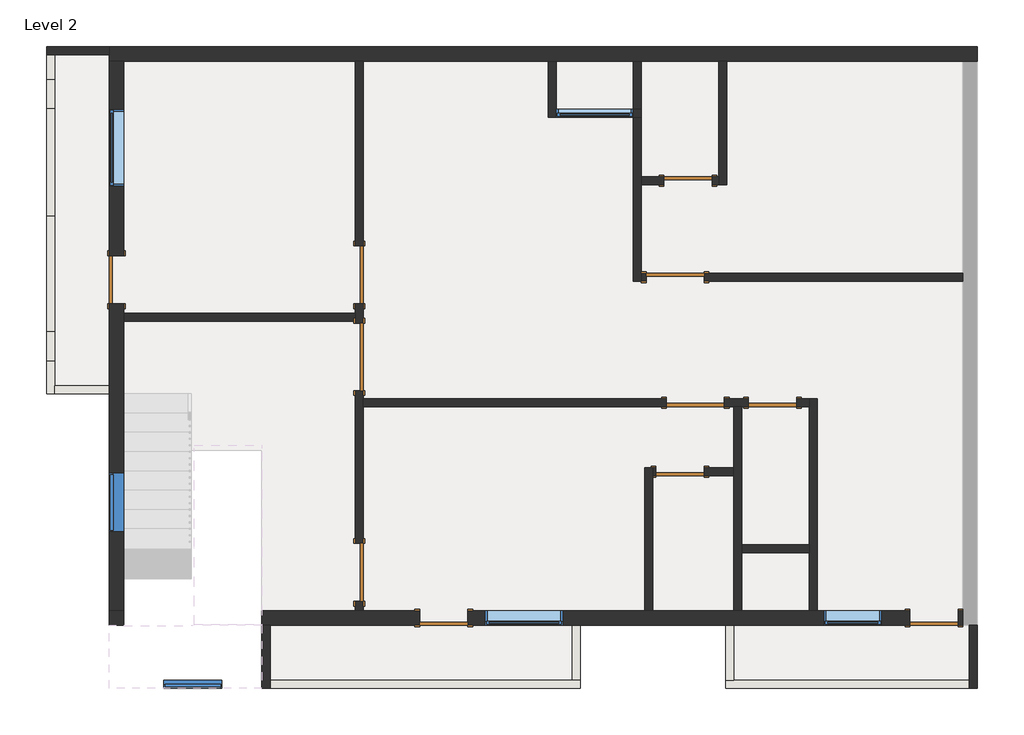
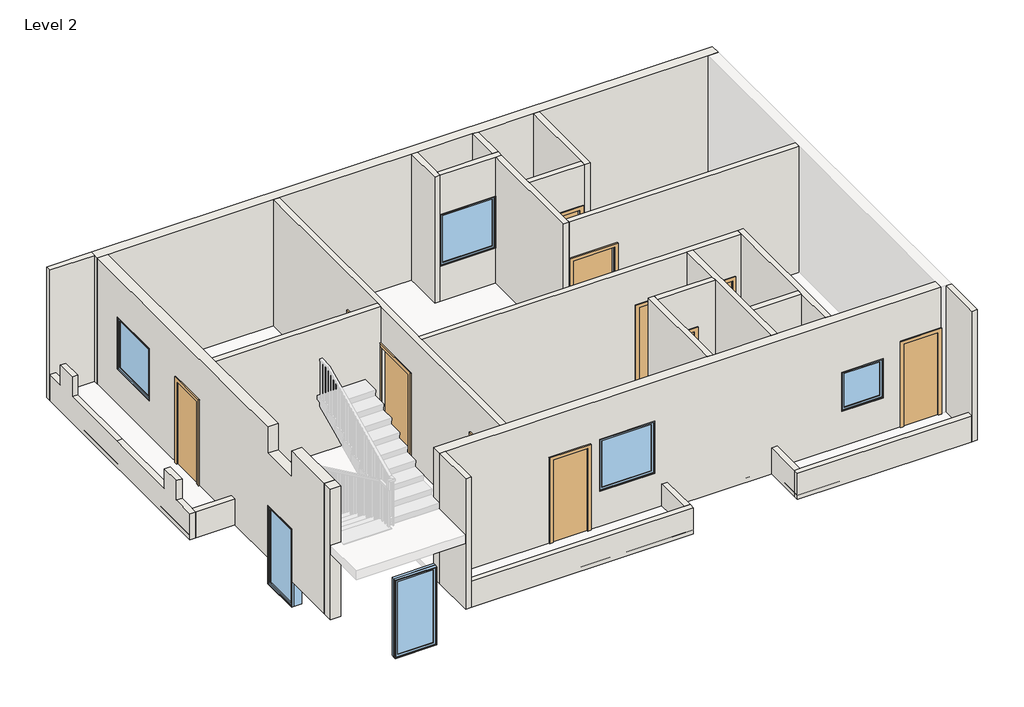
# One storey, part 1 of 2: 28 walls, 11 doors, 6 windows.
"""IFC4 building model written with IfcOpenShell, lengths in millimetres."""

from ifc_helpers import new_model, si_unit, frame, origin, place, context, project, spatial, polyline, outline, extrude, faceted_brep, transform, mapped, element, save
from components import door_1fe7f57d, door_85036156, door_a3eb833a, door_a1797ceb, door_4f94b823, window_6c5853a0, window_7da3115e, window_c796fc87, window_f887c457, window_76f305d9

model = new_model("IFC4")

# Units and contexts
model_context = context("Model", 3, world=origin())
ifc_project = project(units=[si_unit("LENGTHUNIT", "METRE", prefix="MILLI")], contexts=[model_context])

# Site, building, storey
site = spatial("IfcSite", under=ifc_project)
building = spatial("IfcBuilding", under=site)
storey = spatial("IfcBuildingStorey", under=building, Name="Level 2", Elevation=3048.0)

# Doors
placement = place(None, origin())
door_shape = door_1fe7f57d(model_context)
element("IfcDoor", 1, ObjectType="Single-Flush : 30\" x 80\"", at=placement, inside=storey, context=model_context, shape_type="MappedRepresentation", body=[
    mapped(door_shape, transform((-1197.7394758, 10653.5495492, 3048.0), x_axis=(1.0, 0.0, 0.0), y_axis=(0.0, 1.0, 0.0), z_axis=(0.0, 0.0, 1.0))),
])
element("IfcDoor", 2, ObjectType="Single-Flush : 30\" x 80\"", at=placement, inside=storey, context=model_context, shape_type="MappedRepresentation", body=[
    mapped(door_shape, transform((135.7605242, 7148.3495492, 3048.0), x_axis=(-1.0, 0.0, 0.0), y_axis=(0.0, -1.0, 0.0), z_axis=(0.0, 0.0, 1.0))),
])
element("IfcDoor", 3, ObjectType="Single-Flush : 30\" x 80\"", at=placement, inside=storey, context=model_context, shape_type="MappedRepresentation", body=[
    mapped(door_shape, transform((-1324.7394758, 6056.1495492, 3048.0), x_axis=(-1.0, 0.0, 0.0), y_axis=(0.0, -1.0, 0.0), z_axis=(0.0, 0.0, 1.0))),
])
door_2_shape = door_85036156(model_context)
element("IfcDoor", 4, ObjectType="Single-Flush : 30\" x 80\"", at=placement, inside=storey, context=model_context, shape_type="MappedRepresentation", body=[
    mapped(door_2_shape, transform((-10227.4394758, 9091.4495492, 3048.0), x_axis=(0.0, -1.0, 0.0), y_axis=(1.0, 0.0, 0.0), z_axis=(0.0, 0.0, 1.0))),
])
element("IfcDoor", 5, ObjectType="Single-Flush : 30\" x 80\"", at=placement, inside=storey, context=model_context, shape_type="MappedRepresentation", body=[
    mapped(door_2_shape, transform((-5058.5394758, 3744.7495492, 3048.0), x_axis=(1.0, 0.0, 0.0), y_axis=(0.0, 1.0, 0.0), z_axis=(0.0, 0.0, 1.0))),
])
element("IfcDoor", 6, ObjectType="Single-Flush : 30\" x 80\"", at=placement, inside=storey, context=model_context, shape_type="MappedRepresentation", body=[
    mapped(door_2_shape, transform((2688.4605242, 3744.7495492, 3048.0), x_axis=(1.0, 0.0, 0.0), y_axis=(0.0, 1.0, 0.0), z_axis=(0.0, 0.0, 1.0))),
])
door_3_shape = door_a3eb833a(model_context)
element("IfcDoor", 7, ObjectType="Single-Flush : 36\" x 84\"", at=placement, inside=storey, context=model_context, shape_type="MappedRepresentation", body=[
    mapped(door_3_shape, transform((-6392.0394758, 9167.6495492, 3048.0), x_axis=(0.0, 1.0, 0.0), y_axis=(-1.0, 0.0, 0.0), z_axis=(0.0, 0.0, 1.0))),
])
element("IfcDoor", 8, ObjectType="Single-Flush : 36\" x 84\"", at=placement, inside=storey, context=model_context, shape_type="MappedRepresentation", body=[
    mapped(door_3_shape, transform((-1400.9394758, 9129.5495492, 3048.0), x_axis=(-1.0, 0.0, 0.0), y_axis=(0.0, -1.0, 0.0), z_axis=(0.0, 0.0, 1.0))),
])
element("IfcDoor", 9, ObjectType="Single-Flush : 36\" x 84\"", at=placement, inside=storey, context=model_context, shape_type="MappedRepresentation", body=[
    mapped(door_3_shape, transform((-1083.4394758, 7148.3495492, 3048.0), x_axis=(1.0, 0.0, 0.0), y_axis=(0.0, 1.0, 0.0), z_axis=(0.0, 0.0, 1.0))),
])
door_4_shape = door_a1797ceb(model_context)
element("IfcDoor", 10, ObjectType="Single-Flush : 36\" x 84\"", at=placement, inside=storey, context=model_context, shape_type="MappedRepresentation", body=[
    mapped(door_4_shape, transform((-6392.0394758, 4468.6495492, 3048.0), x_axis=(0.0, -1.0, 0.0), y_axis=(1.0, 0.0, 0.0), z_axis=(0.0, 0.0, 1.0))),
])
door_5_shape = door_4f94b823(model_context)
element("IfcDoor", 11, ObjectType="Single-Flush : 42\" x 84\" 3,6\"", at=placement, inside=storey, context=model_context, shape_type="MappedRepresentation", body=[
    mapped(door_5_shape, transform((-6392.0394758, 7872.2495492, 3048.0), x_axis=(0.0, -1.0, 0.0), y_axis=(1.0, 0.0, 0.0), z_axis=(0.0, 0.0, 1.0))),
])

# Walls
element("IfcWall", 12, ObjectType="Generic - 5\"", at=placement, inside=storey, context=model_context, shape_type="Brep", body=[
    faceted_brep([(-6328.5394758, 4925.8495492, 3048.0), (-6328.5394758, 7084.8495492, 3048.0), (-6328.5394758, 7211.8495492, 3048.0), (-6328.5394758, 7338.8495492, 3048.0), (-6328.5394758, 7338.8495492, 5181.6), (-6328.5394758, 8405.6495492, 5181.6), (-6328.5394758, 8405.6495492, 3048.0), (-6328.5394758, 8710.4495492, 3048.0), (-6328.5394758, 8710.4495492, 5181.6), (-6328.5394758, 9624.8495492, 5181.6), (-6328.5394758, 9624.8495492, 3048.0), (-6328.5394758, 12545.8495492, 3048.0), (-6328.5394758, 12545.8495492, 6096.0), (-6328.5394758, 7211.8495492, 6096.0), (-6328.5394758, 7084.8495492, 6096.0), (-6328.5394758, 3859.0495492, 6096.0), (-6328.5394758, 3859.0495492, 3048.0), (-6328.5394758, 4011.4495492, 3048.0), (-6328.5394758, 4011.4495492, 5181.6), (-6328.5394758, 4925.8495492, 5181.6), (-6455.5394758, 7338.8495492, 5181.6), (-6455.5394758, 7338.8495492, 3048.0), (-6455.5394758, 4925.8495492, 3048.0), (-6455.5394758, 4925.8495492, 5181.6), (-6455.5394758, 4011.4495492, 5181.6), (-6455.5394758, 4011.4495492, 3048.0), (-6455.5394758, 3859.0495492, 3048.0), (-6455.5394758, 3859.0495492, 6096.0), (-6455.5394758, 8431.0495492, 6096.0), (-6455.5394758, 8558.0495492, 6096.0), (-6455.5394758, 12545.8495492, 6096.0), (-6455.5394758, 12545.8495492, 3048.0), (-6455.5394758, 9624.8495492, 3048.0), (-6455.5394758, 9624.8495492, 5181.6), (-6455.5394758, 8710.4495492, 5181.6), (-6455.5394758, 8710.4495492, 3048.0), (-6455.5394758, 8558.0495492, 3048.0), (-6455.5394758, 8431.0495492, 3048.0), (-6455.5394758, 8405.6495492, 3048.0), (-6455.5394758, 8405.6495492, 5181.6)], [[[0, 1, 2, 3, 4, 5, 6, 7, 8, 9, 10, 11, 12, 13, 14, 15, 16, 17, 18, 19]], [[20, 21, 22, 23, 24, 25, 26, 27, 28, 29, 30, 31, 32, 33, 34, 35, 36, 37, 38, 39]], [[11, 10, 32, 31]], [[26, 25, 17, 16]], [[22, 21, 3, 2, 1, 0]], [[38, 37, 36, 35, 7, 6]], [[15, 14, 13, 12, 30, 29, 28, 27]], [[16, 15, 27, 26]], [[12, 11, 31, 30]], [[33, 32, 10, 9]], [[34, 33, 9, 8]], [[35, 34, 8, 7]], [[18, 17, 25, 24]], [[19, 18, 24, 23]], [[0, 19, 23, 22]], [[4, 3, 21, 20]], [[5, 4, 20, 39]], [[6, 5, 39, 38]]]),
])
element("IfcWall", 13, ObjectType="Generic - 5\"", at=placement, inside=storey, context=model_context, shape_type="SweptSolid", body=[
    extrude(outline(polyline([(-10113.1394758, 8558.0495492), (-6455.5394758, 8558.0495492), (-6455.5394758, 8431.0495492), (-10113.1394758, 8431.0495492), (-10113.1394758, 8558.0495492)])), frame((0.0, 0.0, 3048.0), z_axis=(0.0, 0.0, 1.0), x_axis=(1.0, 0.0, 0.0)), (0.0, 0.0, 1.0), 3048.0),
])
element("IfcWall", 14, ObjectType="Generic - 5\"", at=placement, inside=storey, context=model_context, shape_type="Brep", body=[
    faceted_brep([(-245.2394758, 7211.8495492, 5080.0), (-245.2394758, 7211.8495492, 3048.0), (-626.2394758, 7211.8495492, 3048.0), (-626.2394758, 7211.8495492, 5181.6), (-1540.6394758, 7211.8495492, 5181.6), (-1540.6394758, 7211.8495492, 3048.0), (-6328.5394758, 7211.8495492, 3048.0), (-6328.5394758, 7211.8495492, 6096.0), (719.9605242, 7211.8495492, 6096.0), (719.9605242, 7211.8495492, 3048.0), (516.7605242, 7211.8495492, 3048.0), (516.7605242, 7211.8495492, 5080.0), (-626.2394758, 7084.8495492, 3048.0), (-473.8394758, 7084.8495492, 3048.0), (-346.8394758, 7084.8495492, 3048.0), (-245.2394758, 7084.8495492, 3048.0), (-245.2394758, 7084.8495492, 5080.0), (516.7605242, 7084.8495492, 5080.0), (516.7605242, 7084.8495492, 3048.0), (719.9605242, 7084.8495492, 3048.0), (719.9605242, 7084.8495492, 6096.0), (-346.8394758, 7084.8495492, 6096.0), (-473.8394758, 7084.8495492, 6096.0), (-6328.5394758, 7084.8495492, 6096.0), (-6328.5394758, 7084.8495492, 3048.0), (-1540.6394758, 7084.8495492, 3048.0), (-1540.6394758, 7084.8495492, 5181.6), (-626.2394758, 7084.8495492, 5181.6)], [[[0, 1, 2, 3, 4, 5, 6, 7, 8, 9, 10, 11]], [[12, 13, 14, 15, 16, 17, 18, 19, 20, 21, 22, 23, 24, 25, 26, 27]], [[25, 24, 6, 5]], [[10, 9, 19, 18]], [[2, 1, 15, 14, 13, 12]], [[8, 7, 23, 22, 21, 20]], [[7, 6, 24, 23]], [[9, 8, 20, 19]], [[3, 2, 12, 27]], [[4, 3, 27, 26]], [[5, 4, 26, 25]], [[16, 15, 1, 0]], [[17, 16, 0, 11]], [[18, 17, 11, 10]]]),
])
element("IfcWall", 15, ObjectType="Generic - 5\"", at=placement, inside=storey, context=model_context, shape_type="Brep", body=[
    faceted_brep([(-2061.3394758, 11656.8495492, 3048.0), (-2061.3394758, 9066.0495492, 3048.0), (-2061.3394758, 9066.0495492, 6096.0), (-2061.3394758, 11656.8495492, 6096.0), (-1934.3394758, 11656.8495492, 3048.0), (-1934.3394758, 11656.8495492, 6096.0), (-1934.3394758, 10717.0495492, 6096.0), (-1934.3394758, 10590.0495492, 6096.0), (-1934.3394758, 9193.0495492, 6096.0), (-1934.3394758, 9066.0495492, 6096.0), (-1934.3394758, 9066.0495492, 3048.0), (-1934.3394758, 9193.0495492, 3048.0), (-1934.3394758, 10590.0495492, 3048.0), (-1934.3394758, 10717.0495492, 3048.0)], [[[0, 1, 2, 3]], [[4, 5, 6, 7, 8, 9, 10, 11, 12, 13]], [[1, 0, 4, 13, 12, 11, 10]], [[3, 2, 9, 8, 7, 6, 5]], [[0, 3, 5, 4]], [[2, 1, 10, 9]]]),
])
element("IfcWall", 16, ObjectType="Generic - 5\"", at=placement, inside=storey, context=model_context, shape_type="SweptSolid", body=[
    extrude(outline(polyline([(3048.0, -1934.3394758), (3048.0, -1858.1394758), (5181.6, -1858.1394758), (5181.6, -943.7394758), (3048.0, -943.7394758), (3048.0, 3145.6605242), (6096.0, 3145.6605242), (6096.0, -1934.3394758), (3048.0, -1934.3394758)])), frame((0.0, 9066.0495492, 0.0), z_axis=(0.0, 1.0, 0.0), x_axis=(0.0, 0.0, 1.0)), (0.0, 0.0, 1.0), 127.0),
])
element("IfcWall", 17, ObjectType="Generic - 5\"", at=placement, inside=storey, context=model_context, shape_type="Brep", body=[
    faceted_brep([(-346.8394758, 3859.0495492, 3048.0), (-346.8394758, 4773.4495492, 3048.0), (-346.8394758, 4900.4495492, 3048.0), (-346.8394758, 7084.8495492, 3048.0), (-346.8394758, 7084.8495492, 6096.0), (-346.8394758, 4900.4495492, 6096.0), (-346.8394758, 4773.4495492, 6096.0), (-346.8394758, 3859.0495492, 6096.0), (-473.8394758, 3859.0495492, 3048.0), (-473.8394758, 3859.0495492, 6096.0), (-473.8394758, 5992.6495492, 6096.0), (-473.8394758, 6119.6495492, 6096.0), (-473.8394758, 7084.8495492, 6096.0), (-473.8394758, 7084.8495492, 3048.0), (-473.8394758, 6119.6495492, 3048.0), (-473.8394758, 5992.6495492, 3048.0)], [[[0, 1, 2, 3, 4, 5, 6, 7]], [[8, 9, 10, 11, 12, 13, 14, 15]], [[3, 2, 1, 0, 8, 15, 14, 13]], [[7, 6, 5, 4, 12, 11, 10, 9]], [[4, 3, 13, 12]], [[0, 7, 9, 8]]]),
])
element("IfcWall", 18, ObjectType="Generic - 5\"", at=placement, inside=storey, context=model_context, shape_type="Brep", body=[
    faceted_brep([(846.9605242, 3859.0495492, 3048.0), (846.9605242, 7211.8495492, 3048.0), (846.9605242, 7211.8495492, 6096.0), (846.9605242, 3859.0495492, 6096.0), (719.9605242, 3859.0495492, 3048.0), (719.9605242, 3859.0495492, 6096.0), (719.9605242, 4773.4495492, 6096.0), (719.9605242, 4900.4495492, 6096.0), (719.9605242, 7084.8495492, 6096.0), (719.9605242, 7211.8495492, 6096.0), (719.9605242, 7211.8495492, 3048.0), (719.9605242, 7084.8495492, 3048.0), (719.9605242, 4900.4495492, 3048.0), (719.9605242, 4773.4495492, 3048.0)], [[[0, 1, 2, 3]], [[4, 5, 6, 7, 8, 9, 10, 11, 12, 13]], [[1, 0, 4, 13, 12, 11, 10]], [[3, 2, 9, 8, 7, 6, 5]], [[0, 3, 5, 4]], [[2, 1, 10, 9]]]),
])
element("IfcWall", 19, ObjectType="Generic - 5\"", at=placement, inside=storey, context=model_context, shape_type="Brep", body=[
    faceted_brep([(-1756.5394758, 3859.0495492, 3048.0), (-1756.5394758, 5992.6495492, 3048.0), (-1756.5394758, 6119.6495492, 3048.0), (-1756.5394758, 6119.6495492, 6096.0), (-1756.5394758, 5992.6495492, 6096.0), (-1756.5394758, 3859.0495492, 6096.0), (-1883.5394758, 3859.0495492, 3048.0), (-1883.5394758, 3859.0495492, 6096.0), (-1883.5394758, 6119.6495492, 6096.0), (-1883.5394758, 6119.6495492, 3048.0)], [[[0, 1, 2, 3, 4, 5]], [[6, 7, 8, 9]], [[2, 1, 0, 6, 9]], [[5, 4, 3, 8, 7]], [[0, 5, 7, 6]], [[3, 2, 9, 8]]]),
])
element("IfcWall", 20, ObjectType="Generic - 5\"", at=placement, inside=storey, context=model_context, shape_type="SweptSolid", body=[
    extrude(outline(polyline([(3048.0, -1756.5394758), (3048.0, -1705.7394758), (5080.0, -1705.7394758), (5080.0, -943.7394758), (3048.0, -943.7394758), (3048.0, -473.8394758), (6096.0, -473.8394758), (6096.0, -1756.5394758), (3048.0, -1756.5394758)])), frame((0.0, 5992.6495492, 0.0), z_axis=(0.0, 1.0, 0.0), x_axis=(0.0, 0.0, 1.0)), (0.0, 0.0, 1.0), 127.0),
])
element("IfcWall", 21, ObjectType="Generic - 5\"", at=placement, inside=storey, context=model_context, shape_type="SweptSolid", body=[
    extrude(outline(polyline([(719.9605242, 4773.4495492), (-346.8394758, 4773.4495492), (-346.8394758, 4900.4495492), (719.9605242, 4900.4495492), (719.9605242, 4773.4495492)])), frame((0.0, 0.0, 3048.0), z_axis=(0.0, 0.0, 1.0), x_axis=(1.0, 0.0, 0.0)), (0.0, 0.0, 1.0), 3048.0),
])
element("IfcWall", 22, ObjectType="Generic - 5\"", at=placement, inside=storey, context=model_context, shape_type="Brep", body=[
    faceted_brep([(-715.1394758, 12545.8495492, 3048.0), (-715.1394758, 10717.0495492, 3048.0), (-715.1394758, 10590.0495492, 3048.0), (-715.1394758, 10590.0495492, 6096.0), (-715.1394758, 10717.0495492, 6096.0), (-715.1394758, 12545.8495492, 6096.0), (-588.1394758, 12545.8495492, 3048.0), (-588.1394758, 12545.8495492, 6096.0), (-588.1394758, 10590.0495492, 6096.0), (-588.1394758, 10590.0495492, 3048.0)], [[[0, 1, 2, 3, 4, 5]], [[6, 7, 8, 9]], [[2, 1, 0, 6, 9]], [[5, 4, 3, 8, 7]], [[0, 5, 7, 6]], [[3, 2, 9, 8]]]),
])
element("IfcWall", 23, ObjectType="Generic - 5\"", at=placement, inside=storey, context=model_context, shape_type="SweptSolid", body=[
    extrude(outline(polyline([(5080.0, -816.7394758), (3048.0, -816.7394758), (3048.0, -715.1394758), (6096.0, -715.1394758), (6096.0, -1934.3394758), (3048.0, -1934.3394758), (3048.0, -1578.7394758), (5080.0, -1578.7394758), (5080.0, -816.7394758)])), frame((0.0, 10590.0495492, 0.0), z_axis=(0.0, 1.0, 0.0), x_axis=(0.0, 0.0, 1.0)), (0.0, 0.0, 1.0), 127.0),
])
element("IfcWall", 24, ObjectType="Generic - 5\"", at=placement, inside=storey, context=model_context, shape_type="Brep", body=[
    faceted_brep([(-3407.5394758, 12545.8495492, 3048.0), (-3407.5394758, 11656.8495492, 3048.0), (-3407.5394758, 11656.8495492, 6096.0), (-3407.5394758, 12545.8495492, 6096.0), (-3280.5394758, 12545.8495492, 3048.0), (-3280.5394758, 12545.8495492, 6096.0), (-3280.5394758, 11783.8495492, 6096.0), (-3280.5394758, 11656.8495492, 6096.0), (-3280.5394758, 11656.8495492, 3048.0), (-3280.5394758, 11783.8495492, 3048.0)], [[[0, 1, 2, 3]], [[4, 5, 6, 7, 8, 9]], [[1, 0, 4, 9, 8]], [[3, 2, 7, 6, 5]], [[0, 3, 5, 4]], [[2, 1, 8, 7]]]),
])
element("IfcWall", 25, ObjectType="Generic - 5\"", at=placement, inside=storey, context=model_context, shape_type="Brep", body=[
    faceted_brep([(-2061.3394758, 11656.8495492, 3962.4), (-3280.5394758, 11656.8495492, 3962.4), (-3280.5394758, 11656.8495492, 3048.0), (-2061.3394758, 11656.8495492, 3048.0), (-1934.3394758, 11656.8495492, 3048.0), (-1934.3394758, 11656.8495492, 6096.0), (-2061.3394758, 11656.8495492, 6096.0), (-3280.5394758, 11656.8495492, 6096.0), (-3280.5394758, 11656.8495492, 5181.6), (-2061.3394758, 11656.8495492, 5181.6), (-3280.5394758, 11783.8495492, 3048.0), (-3280.5394758, 11783.8495492, 3962.4), (-2061.3394758, 11783.8495492, 3962.4), (-2061.3394758, 11783.8495492, 5181.6), (-3280.5394758, 11783.8495492, 5181.6), (-3280.5394758, 11783.8495492, 6096.0), (-2061.3394758, 11783.8495492, 6096.0), (-1934.3394758, 11783.8495492, 6096.0), (-1934.3394758, 11783.8495492, 3048.0), (-2061.3394758, 11783.8495492, 3048.0)], [[[0, 1, 2, 3, 4, 5, 6, 7, 8, 9]], [[10, 11, 12, 13, 14, 15, 16, 17, 18, 19]], [[4, 3, 2, 10, 19, 18]], [[7, 6, 5, 17, 16, 15]], [[8, 7, 15, 14]], [[2, 1, 11, 10]], [[5, 4, 18, 17]], [[12, 11, 1, 0]], [[13, 12, 0, 9]], [[14, 13, 9, 8]]]),
])
element("IfcWall", 26, ObjectType="Generic - 5\"", at=placement, inside=storey, context=model_context, shape_type="SweptSolid", body=[
    extrude(outline(polyline([(-1934.3394758, 12545.8495492), (-1934.3394758, 11783.8495492), (-2061.3394758, 11783.8495492), (-2061.3394758, 12545.8495492), (-1934.3394758, 12545.8495492)])), frame((0.0, 0.0, 3048.0), z_axis=(0.0, 0.0, 1.0), x_axis=(1.0, 0.0, 0.0)), (0.0, 0.0, 1.0), 3048.0),
])
element("IfcWall", 27, ObjectType="Generic - 5\"", at=placement, inside=storey, context=model_context, shape_type="Brep", body=[
    faceted_brep([(3247.2605242, 3630.4495492, 3048.0), (3247.2605242, 2766.8495492, 3048.0), (3247.2605242, 2639.8495492, 3048.0), (3247.2605242, 2639.8495492, 3657.6), (3247.2605242, 2639.8495492, 6096.0), (3247.2605242, 3630.4495492, 6096.0), (3374.2605242, 3630.4495492, 3048.0), (3374.2605242, 3630.4495492, 6096.0), (3374.2605242, 2639.8495492, 6096.0), (3374.2605242, 2639.8495492, 3048.0)], [[[0, 1, 2, 3, 4, 5]], [[6, 7, 8, 9]], [[2, 1, 0, 6, 9]], [[5, 4, 8, 7]], [[0, 5, 7, 6]], [[4, 3, 2, 9, 8]]]),
])
element("IfcWall", 28, ObjectType="Generic - 5\"", at=placement, inside=storey, context=model_context, shape_type="Brep", body=[
    faceted_brep([(3247.2605242, 2766.8495492, 3048.0), (-473.8394758, 2766.8495492, 3048.0), (-600.8394758, 2766.8495492, 3048.0), (-600.8394758, 2766.8495492, 3657.6), (-473.8394758, 2766.8495492, 3657.6), (3247.2605242, 2766.8495492, 3657.6), (3247.2605242, 2639.8495492, 3048.0), (3247.2605242, 2639.8495492, 3657.6), (-600.8394758, 2639.8495492, 3657.6), (-600.8394758, 2639.8495492, 3048.0)], [[[0, 1, 2, 3, 4, 5]], [[6, 7, 8, 9]], [[2, 1, 0, 6, 9]], [[5, 4, 3, 8, 7]], [[0, 5, 7, 6]], [[3, 2, 9, 8]]]),
])
element("IfcWall", 29, ObjectType="Generic - 5\"", at=placement, inside=storey, context=model_context, shape_type="SweptSolid", body=[
    extrude(outline(polyline([(-473.8394758, 3630.4495492), (-473.8394758, 2766.8495492), (-600.8394758, 2766.8495492), (-600.8394758, 3630.4495492), (-473.8394758, 3630.4495492)])), frame((0.0, 0.0, 3048.0), z_axis=(0.0, 0.0, 1.0), x_axis=(1.0, 0.0, 0.0)), (0.0, 0.0, 1.0), 609.6),
])
element("IfcWall", 30, ObjectType="Generic - 5\"", at=placement, inside=storey, context=model_context, shape_type="Brep", body=[
    faceted_brep([(-7928.7394758, 3630.4495492, 3048.0), (-7928.7394758, 2639.8495492, 3048.0), (-7928.7394758, 2639.8495492, 6096.0), (-7928.7394758, 3630.4495492, 6096.0), (-7801.7394758, 3630.4495492, 3048.0), (-7801.7394758, 3630.4495492, 6096.0), (-7801.7394758, 2639.8495492, 6096.0), (-7801.7394758, 2639.8495492, 3657.6), (-7801.7394758, 2639.8495492, 3048.0), (-7801.7394758, 2766.8495492, 3048.0)], [[[0, 1, 2, 3]], [[4, 5, 6, 7, 8, 9]], [[1, 0, 4, 9, 8]], [[3, 2, 6, 5]], [[0, 3, 5, 4]], [[1, 8, 7, 6, 2]]]),
])
element("IfcWall", 31, ObjectType="Generic - 5\"", at=placement, inside=storey, context=model_context, shape_type="Brep", body=[
    faceted_brep([(-7801.7394758, 2639.8495492, 3048.0), (-2899.5394758, 2639.8495492, 3048.0), (-2899.5394758, 2639.8495492, 3657.6), (-7801.7394758, 2639.8495492, 3657.6), (-7801.7394758, 2766.8495492, 3048.0), (-7801.7394758, 2766.8495492, 3657.6), (-3026.5394758, 2766.8495492, 3657.6), (-2899.5394758, 2766.8495492, 3657.6), (-2899.5394758, 2766.8495492, 3048.0), (-3026.5394758, 2766.8495492, 3048.0)], [[[0, 1, 2, 3]], [[4, 5, 6, 7, 8, 9]], [[1, 0, 4, 9, 8]], [[3, 2, 7, 6, 5]], [[2, 1, 8, 7]], [[0, 3, 5, 4]]]),
])
element("IfcWall", 32, ObjectType="Generic - 5\"", at=placement, inside=storey, context=model_context, shape_type="SweptSolid", body=[
    extrude(outline(polyline([(-2899.5394758, 3630.4495492), (-2899.5394758, 2766.8495492), (-3026.5394758, 2766.8495492), (-3026.5394758, 3630.4495492), (-2899.5394758, 3630.4495492)])), frame((0.0, 0.0, 3048.0), z_axis=(0.0, 0.0, 1.0), x_axis=(1.0, 0.0, 0.0)), (0.0, 0.0, 1.0), 609.6),
])
element("IfcWall", 33, ObjectType="Generic - 5\"", at=placement, inside=storey, context=model_context, shape_type="Brep", body=[
    faceted_brep([(-10341.7394758, 12774.4495492, 3048.0), (-11332.3394758, 12774.4495492, 3048.0), (-11332.3394758, 12774.4495492, 6096.0), (-10341.7394758, 12774.4495492, 6096.0), (-10341.7394758, 12647.4495492, 3048.0), (-10341.7394758, 12647.4495492, 6096.0), (-11332.3394758, 12647.4495492, 6096.0), (-11332.3394758, 12647.4495492, 3657.6), (-11332.3394758, 12647.4495492, 3048.0), (-11205.3394758, 12647.4495492, 3048.0)], [[[0, 1, 2, 3]], [[4, 5, 6, 7, 8, 9]], [[1, 0, 4, 9, 8]], [[3, 2, 6, 5]], [[0, 3, 5, 4]], [[2, 1, 8, 7, 6]]]),
])
element("IfcWall", 34, ObjectType="Generic - 5\"", at=placement, inside=storey, context=model_context, shape_type="Brep", body=[
    faceted_brep([(-11332.3394758, 12647.4495492, 3048.0), (-11332.3394758, 7288.0495492, 3048.0), (-11332.3394758, 7288.0495492, 3657.6), (-11332.3394758, 7808.7495492, 3657.6), (-11332.3394758, 7808.7495492, 4114.8), (-11332.3394758, 8265.9495492, 4114.8), (-11332.3394758, 8265.9495492, 3657.6), (-11332.3394758, 10094.7495492, 3657.6), (-11332.3394758, 11796.5495492, 3657.6), (-11332.3394758, 11796.5495492, 4114.8), (-11332.3394758, 12253.7495492, 4114.8), (-11332.3394758, 12253.7495492, 3657.6), (-11332.3394758, 12647.4495492, 3657.6), (-11205.3394758, 12647.4495492, 3048.0), (-11205.3394758, 12647.4495492, 3657.6), (-11205.3394758, 12253.7495492, 3657.6), (-11205.3394758, 12253.7495492, 4114.8), (-11205.3394758, 11796.5495492, 4114.8), (-11205.3394758, 11796.5495492, 3657.6), (-11205.3394758, 10094.7495492, 3657.6), (-11205.3394758, 8265.9495492, 3657.6), (-11205.3394758, 8265.9495492, 4114.8), (-11205.3394758, 7808.7495492, 4114.8), (-11205.3394758, 7808.7495492, 3657.6), (-11205.3394758, 7415.0495492, 3657.6), (-11205.3394758, 7288.0495492, 3657.6), (-11205.3394758, 7288.0495492, 3048.0), (-11205.3394758, 7415.0495492, 3048.0)], [[[0, 1, 2, 3, 4, 5, 6, 7, 8, 9, 10, 11, 12]], [[13, 14, 15, 16, 17, 18, 19, 20, 21, 22, 23, 24, 25, 26, 27]], [[0, 12, 14, 13]], [[2, 1, 26, 25]], [[1, 0, 13, 27, 26]], [[3, 2, 25, 24, 23]], [[4, 3, 23, 22]], [[5, 4, 22, 21]], [[6, 5, 21, 20]], [[7, 6, 20, 19]], [[8, 7, 19, 18]], [[9, 8, 18, 17]], [[10, 9, 17, 16]], [[11, 10, 16, 15]], [[12, 11, 15, 14]]]),
])
element("IfcWall", 35, ObjectType="Generic - 5\"", at=placement, inside=storey, context=model_context, shape_type="SweptSolid", body=[
    extrude(outline(polyline([(-10341.7394758, 7288.0495492), (-11205.3394758, 7288.0495492), (-11205.3394758, 7415.0495492), (-10341.7394758, 7415.0495492), (-10341.7394758, 7288.0495492)])), frame((0.0, 0.0, 3048.0), z_axis=(0.0, 0.0, 1.0), x_axis=(1.0, 0.0, 0.0)), (0.0, 0.0, 1.0), 609.6),
])
element("IfcWall", 36, ObjectType="Generic - 9\"", at=placement, inside=storey, context=model_context, shape_type="Brep", body=[
    faceted_brep([(-10341.7394758, 12545.8495492, 3048.0), (-10113.1394758, 12545.8495492, 3048.0), (-6455.5394758, 12545.8495492, 3048.0), (-6328.5394758, 12545.8495492, 3048.0), (-3407.5394758, 12545.8495492, 3048.0), (-3280.5394758, 12545.8495492, 3048.0), (-2061.3394758, 12545.8495492, 3048.0), (-1934.3394758, 12545.8495492, 3048.0), (-715.1394758, 12545.8495492, 3048.0), (-588.1394758, 12545.8495492, 3048.0), (3145.6605242, 12545.8495492, 3048.0), (3374.2605242, 12545.8495492, 3048.0), (3374.2605242, 12545.8495492, 6096.0), (3145.6605242, 12545.8495492, 6096.0), (-588.1394758, 12545.8495492, 6096.0), (-715.1394758, 12545.8495492, 6096.0), (-1934.3394758, 12545.8495492, 6096.0), (-2061.3394758, 12545.8495492, 6096.0), (-3280.5394758, 12545.8495492, 6096.0), (-3407.5394758, 12545.8495492, 6096.0), (-6328.5394758, 12545.8495492, 6096.0), (-6455.5394758, 12545.8495492, 6096.0), (-10113.1394758, 12545.8495492, 6096.0), (-10341.7394758, 12545.8495492, 6096.0), (-10341.7394758, 12774.4495492, 3048.0), (-10341.7394758, 12774.4495492, 6096.0), (3374.2605242, 12774.4495492, 6096.0), (3374.2605242, 12774.4495492, 3048.0), (-10341.7394758, 12647.4495492, 3048.0), (-10341.7394758, 12647.4495492, 6096.0)], [[[0, 1, 2, 3, 4, 5, 6, 7, 8, 9, 10, 11, 12, 13, 14, 15, 16, 17, 18, 19, 20, 21, 22, 23]], [[24, 25, 26, 27]], [[11, 10, 9, 8, 7, 6, 5, 4, 3, 2, 1, 0, 28, 24, 27]], [[23, 22, 21, 20, 19, 18, 17, 16, 15, 14, 13, 12, 26, 25, 29]], [[12, 11, 27, 26]], [[0, 23, 29, 25, 24, 28]]]),
])
element("IfcWall", 37, ObjectType="Generic - 9\"", at=placement, inside=storey, context=model_context, shape_type="Brep", body=[
    faceted_brep([(3145.6605242, 3859.0495492, 3048.0), (3069.4605242, 3859.0495492, 3048.0), (3069.4605242, 3859.0495492, 5080.0), (2307.4605242, 3859.0495492, 5080.0), (2307.4605242, 3859.0495492, 3048.0), (846.9605242, 3859.0495492, 3048.0), (719.9605242, 3859.0495492, 3048.0), (-346.8394758, 3859.0495492, 3048.0), (-473.8394758, 3859.0495492, 3048.0), (-1756.5394758, 3859.0495492, 3048.0), (-1883.5394758, 3859.0495492, 3048.0), (-4677.5394758, 3859.0495492, 3048.0), (-4677.5394758, 3859.0495492, 5080.0), (-5439.5394758, 3859.0495492, 5080.0), (-5439.5394758, 3859.0495492, 3048.0), (-6328.5394758, 3859.0495492, 3048.0), (-6455.5394758, 3859.0495492, 3048.0), (-7928.7394758, 3859.0495492, 3048.0), (-7928.7394758, 3859.0495492, 6096.0), (-6455.5394758, 3859.0495492, 6096.0), (-6328.5394758, 3859.0495492, 6096.0), (-1883.5394758, 3859.0495492, 6096.0), (-1756.5394758, 3859.0495492, 6096.0), (-473.8394758, 3859.0495492, 6096.0), (-346.8394758, 3859.0495492, 6096.0), (719.9605242, 3859.0495492, 6096.0), (846.9605242, 3859.0495492, 6096.0), (3145.6605242, 3859.0495492, 6096.0), (-4398.1394758, 3859.0495492, 5181.6), (-4398.1394758, 3859.0495492, 3962.4), (-3178.9394758, 3859.0495492, 3962.4), (-3178.9394758, 3859.0495492, 5181.6), (948.5605242, 3859.0495492, 4876.8), (948.5605242, 3859.0495492, 3962.4), (1862.9605242, 3859.0495492, 3962.4), (1862.9605242, 3859.0495492, 4876.8), (3069.4605242, 3630.4495492, 5080.0), (3069.4605242, 3630.4495492, 3048.0), (3145.6605242, 3630.4495492, 3048.0), (3145.6605242, 3630.4495492, 6096.0), (-7801.7394758, 3630.4495492, 6096.0), (-7928.7394758, 3630.4495492, 6096.0), (-7928.7394758, 3630.4495492, 3048.0), (-7801.7394758, 3630.4495492, 3048.0), (-5439.5394758, 3630.4495492, 3048.0), (-5439.5394758, 3630.4495492, 5080.0), (-4677.5394758, 3630.4495492, 5080.0), (-4677.5394758, 3630.4495492, 3048.0), (-3026.5394758, 3630.4495492, 3048.0), (-2899.5394758, 3630.4495492, 3048.0), (-600.8394758, 3630.4495492, 3048.0), (-473.8394758, 3630.4495492, 3048.0), (2307.4605242, 3630.4495492, 3048.0), (2307.4605242, 3630.4495492, 5080.0), (-4398.1394758, 3630.4495492, 5181.6), (-3178.9394758, 3630.4495492, 5181.6), (-3178.9394758, 3630.4495492, 3962.4), (-4398.1394758, 3630.4495492, 3962.4), (948.5605242, 3630.4495492, 4876.8), (1862.9605242, 3630.4495492, 4876.8), (1862.9605242, 3630.4495492, 3962.4), (948.5605242, 3630.4495492, 3962.4)], [[[0, 1, 2, 3, 4, 5, 6, 7, 8, 9, 10, 11, 12, 13, 14, 15, 16, 17, 18, 19, 20, 21, 22, 23, 24, 25, 26, 27], [28, 29, 30, 31], [32, 33, 34, 35]], [[36, 37, 38, 39, 40, 41, 42, 43, 44, 45, 46, 47, 48, 49, 50, 51, 52, 53], [54, 55, 56, 57], [58, 59, 60, 61]], [[44, 43, 42, 17, 16, 15, 14]], [[38, 37, 1, 0]], [[52, 51, 50, 49, 48, 47, 11, 10, 9, 8, 7, 6, 5, 4]], [[27, 26, 25, 24, 23, 22, 21, 20, 19, 18, 41, 40, 39]], [[0, 27, 39, 38]], [[18, 17, 42, 41]], [[29, 28, 54, 57]], [[30, 29, 57, 56]], [[31, 30, 56, 55]], [[28, 31, 55, 54]], [[12, 11, 47, 46]], [[13, 12, 46, 45]], [[14, 13, 45, 44]], [[2, 1, 37, 36]], [[3, 2, 36, 53]], [[4, 3, 53, 52]], [[33, 32, 58, 61]], [[34, 33, 61, 60]], [[35, 34, 60, 59]], [[32, 35, 59, 58]]]),
])
element("IfcWall", 38, ObjectType="Generic - 9\"", at=placement, inside=storey, context=model_context, shape_type="Brep", body=[
    faceted_brep([(-10113.1394758, 12545.8495492, 3048.0), (-10113.1394758, 12545.8495492, 6096.0), (-10113.1394758, 8558.0495492, 6096.0), (-10113.1394758, 8431.0495492, 6096.0), (-10113.1394758, 7351.5495492, 6096.0), (-10113.1394758, 6030.7495492, 6096.0), (-10113.1394758, 6030.7495492, 5486.4), (-10113.1394758, 5116.3495492, 5486.4), (-10113.1394758, 5116.3495492, 6096.0), (-10113.1394758, 3859.0495492, 6096.0), (-10113.1394758, 3859.0495492, 3048.0), (-10113.1394758, 5116.3495492, 3048.0), (-10113.1394758, 5116.3495492, 4267.2), (-10113.1394758, 6030.7495492, 4267.2), (-10113.1394758, 6030.7495492, 3048.0), (-10113.1394758, 8431.0495492, 3048.0), (-10113.1394758, 8558.0495492, 3048.0), (-10113.1394758, 8710.4495492, 3048.0), (-10113.1394758, 8710.4495492, 5080.0), (-10113.1394758, 9472.4495492, 5080.0), (-10113.1394758, 9472.4495492, 3048.0), (-10113.1394758, 11783.8495492, 5181.6), (-10113.1394758, 11783.8495492, 3962.4), (-10113.1394758, 10564.6495492, 3962.4), (-10113.1394758, 10564.6495492, 5181.6), (-10341.7394758, 12545.8495492, 6096.0), (-10341.7394758, 12545.8495492, 3048.0), (-10341.7394758, 9472.4495492, 3048.0), (-10341.7394758, 9472.4495492, 5080.0), (-10341.7394758, 8710.4495492, 5080.0), (-10341.7394758, 8710.4495492, 3048.0), (-10341.7394758, 7415.0495492, 3048.0), (-10341.7394758, 7288.0495492, 3048.0), (-10341.7394758, 6030.7495492, 3048.0), (-10341.7394758, 6030.7495492, 4267.2), (-10341.7394758, 5116.3495492, 4267.2), (-10341.7394758, 5116.3495492, 3048.0), (-10341.7394758, 3859.0495492, 3048.0), (-10341.7394758, 3859.0495492, 6096.0), (-10341.7394758, 5116.3495492, 6096.0), (-10341.7394758, 5116.3495492, 5486.4), (-10341.7394758, 6030.7495492, 5486.4), (-10341.7394758, 6030.7495492, 6096.0), (-10341.7394758, 7351.5495492, 6096.0), (-10341.7394758, 11783.8495492, 5181.6), (-10341.7394758, 10564.6495492, 5181.6), (-10341.7394758, 10564.6495492, 3962.4), (-10341.7394758, 11783.8495492, 3962.4)], [[[0, 1, 2, 3, 4, 5, 6, 7, 8, 9, 10, 11, 12, 13, 14, 15, 16, 17, 18, 19, 20], [21, 22, 23, 24]], [[25, 26, 27, 28, 29, 30, 31, 32, 33, 34, 35, 36, 37, 38, 39, 40, 41, 42, 43], [44, 45, 46, 47]], [[26, 0, 20, 27]], [[10, 37, 36, 11]], [[30, 17, 16, 15, 14, 33, 32, 31]], [[1, 25, 43, 42, 5, 4, 3, 2]], [[38, 9, 8, 39]], [[1, 0, 26, 25]], [[10, 9, 38, 37]], [[22, 21, 44, 47]], [[23, 22, 47, 46]], [[24, 23, 46, 45]], [[21, 24, 45, 44]], [[18, 17, 30, 29]], [[19, 18, 29, 28]], [[20, 19, 28, 27]], [[13, 34, 33, 14]], [[35, 12, 11, 36]], [[34, 13, 12, 35]], [[41, 6, 5, 42]], [[6, 41, 40, 7]], [[7, 40, 39, 8]]]),
])
element("IfcWall", 39, ObjectType="Generic - 9\"", at=placement, inside=storey, context=model_context, shape_type="SweptSolid", body=[
    extrude(outline(polyline([(-10341.7394758, 3859.0495492), (-10113.1394758, 3859.0495492), (-10113.1394758, 3630.4495492), (-10341.7394758, 3630.4495492), (-10341.7394758, 3859.0495492)])), frame((0.0, 0.0, 3048.0), z_axis=(0.0, 0.0, 1.0), x_axis=(1.0, 0.0, 0.0)), (0.0, 0.0, 1.0), 3048.0),
])

# Windows
window_shape = window_6c5853a0(model_context)
element("IfcWindow", 40, ObjectType="Fixed : 36\" x 36\"", at=placement, inside=storey, context=model_context, shape_type="MappedRepresentation", body=[
    mapped(window_shape, transform((1367.6605242, 3744.7495492, 3048.0), x_axis=(-1.0, 0.0, 0.0), y_axis=(0.0, -1.0, 0.0), z_axis=(0.0, 0.0, 1.0))),
])
window_2_shape = window_7da3115e(model_context)
element("IfcWindow", 41, ObjectType="Fixed : 36\" x 72\"", at=placement, inside=storey, context=model_context, shape_type="MappedRepresentation", body=[
    mapped(window_2_shape, transform((-9059.0394758, 2703.3495492, 2133.6), x_axis=(-1.0, 0.0, 0.0), y_axis=(0.0, -1.0, 0.0), z_axis=(0.0, 0.0, 1.0))),
])
window_3_shape = window_c796fc87(model_context)
element("IfcWindow", 42, ObjectType="Fixed : 36\" x 72\"", at=placement, inside=storey, context=model_context, shape_type="MappedRepresentation", body=[
    mapped(window_3_shape, transform((-10227.4394758, 5611.6495492, 2133.6), x_axis=(0.0, 1.0, 0.0), y_axis=(-1.0, 0.0, 0.0), z_axis=(0.0, 0.0, 1.0))),
])
window_4_shape = window_f887c457(model_context)
element("IfcWindow", 43, ObjectType="Fixed : 48\" x 48\"", at=placement, inside=storey, context=model_context, shape_type="MappedRepresentation", body=[
    mapped(window_4_shape, transform((-2709.0394758, 11720.3495492, 3048.0), x_axis=(-1.0, 0.0, 0.0), y_axis=(0.0, -1.0, 0.0), z_axis=(0.0, 0.0, 1.0))),
])
window_5_shape = window_76f305d9(model_context)
element("IfcWindow", 44, ObjectType="Fixed : 48\" x 48\"", at=placement, inside=storey, context=model_context, shape_type="MappedRepresentation", body=[
    mapped(window_5_shape, transform((-10227.4394758, 11212.3495492, 3048.0), x_axis=(0.0, 1.0, 0.0), y_axis=(-1.0, 0.0, 0.0), z_axis=(0.0, 0.0, 1.0))),
])
element("IfcWindow", 45, ObjectType="Fixed : 48\" x 48\"", at=placement, inside=storey, context=model_context, shape_type="MappedRepresentation", body=[
    mapped(window_5_shape, transform((-3826.6394758, 3744.7495492, 3048.0), x_axis=(-1.0, 0.0, 0.0), y_axis=(0.0, -1.0, 0.0), z_axis=(0.0, 0.0, 1.0))),
])

save(model, "model.ifc")

# Revit data of these elements
# Type "Single-Flush : 30\" x 80\""
#   Type Mark = "5"
#   Assembly Code = "C1020"
#   Thickness = 0' - 2"
#   Height = 6' - 8"
#   Trim Projection Ext = 0' - 1"
#   Trim Projection Int = 0' - 1"
#   Trim Width = 0' - 3"
#   Width = 2' - 6"
#   Door Material = Door - Panel
#   Frame Material = Door - Frame
#   Function = (empty or 0)
#   Wall Closure = (empty or 0)
# Type "Single-Flush : 36\" x 84\""
#   Type Mark = "1"
#   Assembly Code = "C1020"
#   Thickness = 0' - 2"
#   Height = 7' - 0"
#   Trim Projection Ext = 0' - 1"
#   Trim Projection Int = 0' - 1"
#   Trim Width = 0' - 3"
#   Width = 3' - 0"
#   Door Material = Door - Panel
#   Frame Material = Door - Frame
#   Function = (empty or 0)
#   Wall Closure = (empty or 0)
# Type "Single-Flush : 42\" x 84\" 3,6\""
#   Type Mark = "8"
#   Assembly Code = "C1020"
#   Thickness = 0' - 2"
#   Height = 7' - 0"
#   Trim Projection Ext = 0' - 1"
#   Trim Projection Int = 0' - 1"
#   Trim Width = 0' - 3"
#   Width = 3' - 6"
#   Door Material = Door - Panel
#   Frame Material = Door - Frame
#   Function = (empty or 0)
#   Wall Closure = (empty or 0)
# Type "Generic - 5\""
#   Assembly Code = "B2010"
#   Layers, outside or top first: 0' - 5" no material (function 1)
# Type "Generic - 9\""
#   Assembly Code = "B2010"
#   Layers, outside or top first: 0' - 9" no material (function 1)
# Type "Fixed : 36\" x 36\""
#   Type Mark = "4"
#   Assembly Code = "B2020100"
#   Height = 3' - 0"
#   Default Sill Height = 3' - 0"
#   Width = 3' - 0"
#   Window Inset = 0' - 0 3/4"
#   Glass Pane Material = Glass
#   Sash Material = Sash
#   Wall Closure = (empty or 0)
# Type "Fixed : 36\" x 72\""
#   Type Mark = "9"
#   Assembly Code = "B2020100"
#   Height = 6' - 0"
#   Default Sill Height = 1' - 0"
#   Width = 3' - 0"
#   Window Inset = 0' - 0 3/4"
#   Glass Pane Material = Glass
#   Sash Material = Sash
#   Wall Closure = (empty or 0)
# Type "Fixed : 48\" x 48\""
#   Type Mark = "2"
#   Assembly Code = "B2020100"
#   Height = 4' - 0"
#   Default Sill Height = 3' - 0"
#   Width = 4' - 0"
#   Window Inset = 0' - 0 3/4"
#   Glass Pane Material = Glass
#   Sash Material = Sash
#   Wall Closure = (empty or 0)
# Elements 1, 2, 3, 4, 5, 6 (IfcDoor, "Single-Flush : 30\" x 80\"")
#   Phase Created = New Construction
#   Materials on its faces: "Door - Frame", "Door - Panel"
# Elements 7, 8, 9, 10 (IfcDoor, "Single-Flush : 36\" x 84\"")
#   Phase Created = New Construction
#   Materials on its faces: "Door - Frame", "Door - Panel"
# Element 11 (IfcDoor, "Single-Flush : 42\" x 84\" 3,6\"")
#   Phase Created = New Construction
#   Materials on its faces: "Door - Frame", "Door - Panel"
# Elements 12, 13, 14, 15, 16, 17, 18, 19, 20, 21, 22, 23, 24, 25, 26 (IfcWall, "Generic - 5\"")
#   Top Offset = 0' - 0"
#   Base Offset = 0' - 0"
#   Unconnected Height = 10' - 0"
#   wall height = 10' - 0"
#   Phase Created = New Construction
#   Base Constraint = Level 2
#   Materials on its faces: "Default Wall"
# Elements 27, 33 (IfcWall, "Generic - 5\"")
#   Top Offset = 0' - 0"
#   Base Offset = 0' - 0"
#   Unconnected Height = 10' - 0"
#   wall height = 10' - 0"
#   Phase Created = New Construction
#   Base Constraint = Level 2
#   Materials on its faces: "Default Wall", "02 white", "01 colour 1"
# Elements 28, 29, 31, 32 (IfcWall, "Generic - 5\"")
#   Top Offset = 0' - 0"
#   Base Offset = 0' - 0"
#   Unconnected Height = 2' - 0"
#   wall height = 2' - 0"
#   Phase Created = New Construction
#   Base Constraint = Level 2
#   Materials on its faces: "Default Wall", "02 white"
# Element 30 (IfcWall, "Generic - 5\"")
#   Top Offset = 0' - 0"
#   Base Offset = 0' - 0"
#   Unconnected Height = 10' - 0"
#   wall height = 10' - 0"
#   Phase Created = New Construction
#   Base Constraint = Level 2
#   Materials on its faces: "Default Wall", "02 white"
# Elements 34, 35 (IfcWall, "Generic - 5\"")
#   Top Offset = 0' - 0"
#   Base Offset = 0' - 0"
#   Unconnected Height = 2' - 0"
#   wall height = 2' - 0"
#   Phase Created = New Construction
#   Base Constraint = Level 2
#   Materials on its faces: "Default Wall", "01 colour 1"
# Element 36 (IfcWall, "Generic - 9\"")
#   Top Offset = 0' - 0"
#   Base Offset = 0' - 0"
#   Unconnected Height = 10' - 0"
#   wall height = 10' - 0"
#   Phase Created = New Construction
#   Base Constraint = Level 2
#   Materials on its faces: "Default Wall", "02 white", "01 colour 1"
# Elements 37, 38, 39 (IfcWall, "Generic - 9\"")
#   Top Offset = 0' - 0"
#   Base Offset = 0' - 0"
#   Unconnected Height = 10' - 0"
#   wall height = 10' - 0"
#   Phase Created = New Construction
#   Base Constraint = Level 2
#   Materials on its faces: "Default Wall", "01 colour 1"
# Element 40 (IfcWindow, "Fixed : 36\" x 36\"")
#   Mark = "15"
#   Phase Created = New Construction
#   Materials on its faces: "Sash", "Glass"
# Element 41 (IfcWindow, "Fixed : 36\" x 72\"")
#   Mark = "4"
#   Phase Created = New Construction
#   Materials on its faces: "Sash", "Glass"
# Element 42 (IfcWindow, "Fixed : 36\" x 72\"")
#   Mark = "18"
#   Phase Created = New Construction
#   Materials on its faces: "Sash", "Glass"
# Element 43 (IfcWindow, "Fixed : 48\" x 48\"")
#   Mark = "2"
#   Phase Created = New Construction
#   Materials on its faces: "Sash", "Glass"
# Element 44 (IfcWindow, "Fixed : 48\" x 48\"")
#   Mark = "8"
#   Phase Created = New Construction
#   Materials on its faces: "Sash", "Glass"
# Element 45 (IfcWindow, "Fixed : 48\" x 48\"")
#   Mark = "9"
#   Phase Created = New Construction
#   Materials on its faces: "Sash", "Glass"
# Materials
#   "Door - Panel": class "Wood", colour RGB 114 82 51, transparency 0
#   "Door - Frame": colour RGB 153 76 43, transparency 0
#   "Glass": class "Glass", colour RGB 218 227 224, transparency 0.85, Description = "Soda Lime Glass", Cost = 0
#   "Sash": class "Wood", colour RGB 136 99 55, transparency 0
#   "Default Wall": colour RGB 80 80 80, transparency 0
#   "02 white": class "Generic", colour RGB 120 120 120, transparency 0, Cost = 0
#   "01 colour 1": class "Generic", colour RGB 120 120 120, transparency 0, Cost = 0
